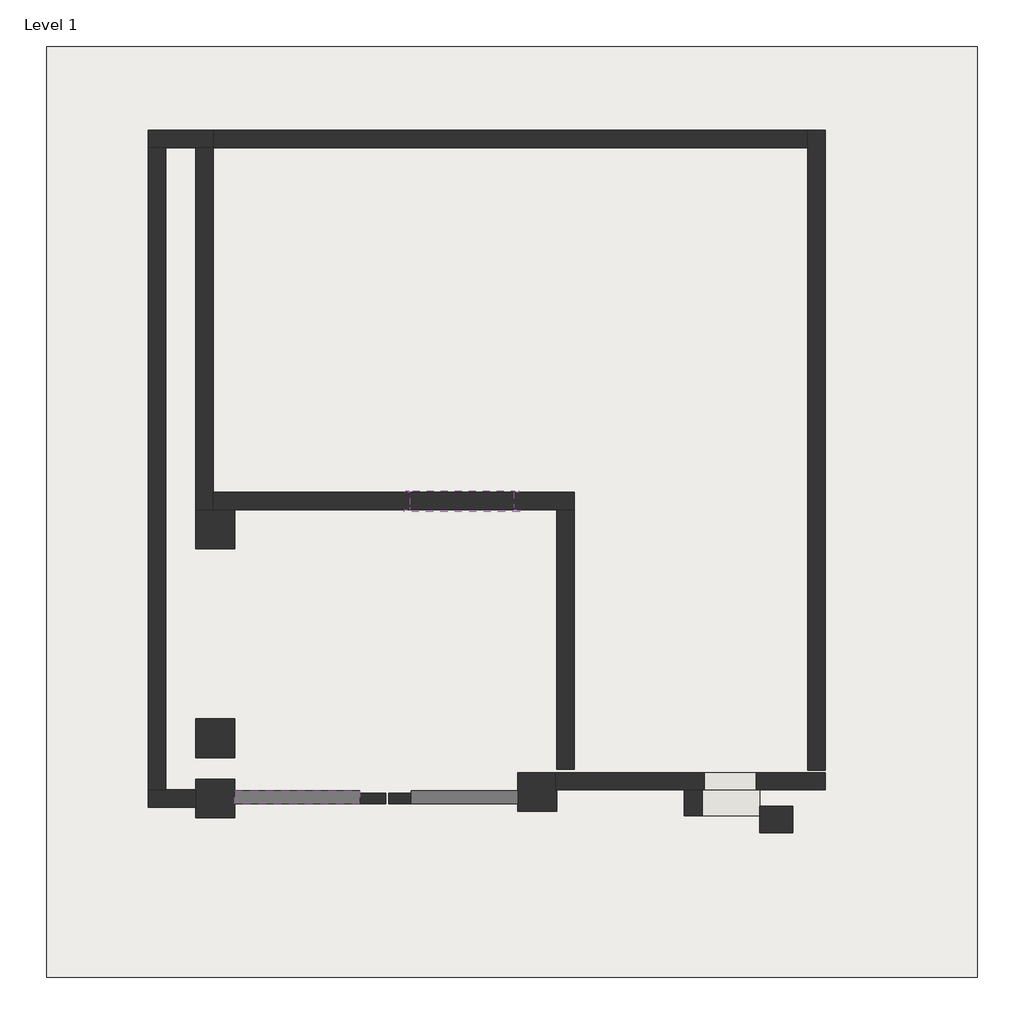
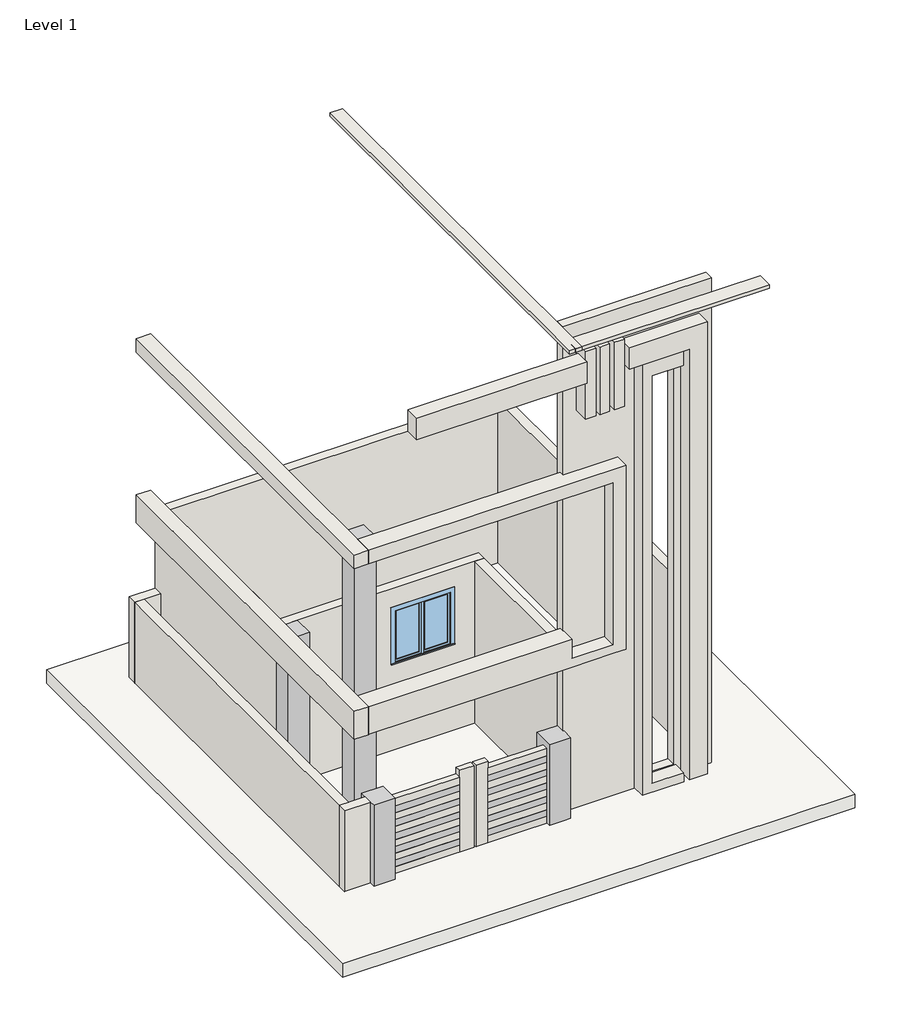
# One storey: 12 walls, 5 proxies, 4 columns, 1 slab, 1 window.
"""IFC4 building model written with IfcOpenShell, lengths in millimetres."""

from ifc_helpers import new_model, si_unit, frame, origin, origin_with_axes, place, context, project, spatial, polyline, outline, extrude, faceted_brep, transform, mapped, element, save
from components import column_b90849dc, walls_1_walls_1_d3114a13, window_0862ab64

model = new_model("IFC4")

# Units and contexts
model_context = context("Model", 3, world=origin())
ifc_project = project(units=[si_unit("LENGTHUNIT", "METRE", prefix="MILLI")], contexts=[model_context])

# Site, building, storey
site = spatial("IfcSite", under=ifc_project)
building = spatial("IfcBuilding", under=site)
storey = spatial("IfcBuildingStorey", under=building, Name="Level 1", Elevation=0.0)

# Proxies
placement = place(None, origin())
element("IfcBuildingElementProxy", 1, Name="Reveal", ObjectType="Reveal", at=placement, inside=storey, context=model_context, shape_type="SweptSolid", body=[
    extrude(outline(polyline([(-7157.3125658, 3805.6483979), (-7157.3125658, 3958.0483979), (-5684.1125658, 3958.0483979), (-5684.1125658, 3805.6483979), (-7157.3125658, 3805.6483979)])), frame((0.0, 0.0, 1371.6), z_axis=(0.0, 0.0, 1.0), x_axis=(1.0, 0.0, 0.0)), (0.0, 0.0, 1.0), 152.4),
    extrude(outline(polyline([(-5074.5125658, 3805.6483979), (-5074.5125658, 3958.0483979), (-3817.2125658, 3958.0483979), (-3817.2125658, 3805.6483979), (-5074.5125658, 3805.6483979)])), frame((0.0, 0.0, 1371.6), z_axis=(0.0, 0.0, 1.0), x_axis=(1.0, 0.0, 0.0)), (0.0, 0.0, 1.0), 152.4),
])
element("IfcBuildingElementProxy", 2, Name="Reveal", ObjectType="Reveal", at=placement, inside=storey, context=model_context, shape_type="SweptSolid", body=[
    extrude(outline(polyline([(-7157.3125658, 3805.6483979), (-7157.3125658, 3958.0483979), (-5684.1125658, 3958.0483979), (-5684.1125658, 3805.6483979), (-7157.3125658, 3805.6483979)])), frame((0.0, 0.0, 1066.8), z_axis=(0.0, 0.0, 1.0), x_axis=(1.0, 0.0, 0.0)), (0.0, 0.0, 1.0), 152.4),
    extrude(outline(polyline([(-5074.5125658, 3805.6483979), (-5074.5125658, 3958.0483979), (-3817.2125658, 3958.0483979), (-3817.2125658, 3805.6483979), (-5074.5125658, 3805.6483979)])), frame((0.0, 0.0, 1066.8), z_axis=(0.0, 0.0, 1.0), x_axis=(1.0, 0.0, 0.0)), (0.0, 0.0, 1.0), 152.4),
])
element("IfcBuildingElementProxy", 3, Name="Reveal", ObjectType="Reveal", at=placement, inside=storey, context=model_context, shape_type="SweptSolid", body=[
    extrude(outline(polyline([(-7157.3125658, 3805.6483979), (-7157.3125658, 3958.0483979), (-5684.1125658, 3958.0483979), (-5684.1125658, 3805.6483979), (-7157.3125658, 3805.6483979)])), frame((0.0, 0.0, 762.0), z_axis=(0.0, 0.0, 1.0), x_axis=(1.0, 0.0, 0.0)), (0.0, 0.0, 1.0), 152.4),
    extrude(outline(polyline([(-5074.5125658, 3805.6483979), (-5074.5125658, 3958.0483979), (-3817.2125658, 3958.0483979), (-3817.2125658, 3805.6483979), (-5074.5125658, 3805.6483979)])), frame((0.0, 0.0, 762.0), z_axis=(0.0, 0.0, 1.0), x_axis=(1.0, 0.0, 0.0)), (0.0, 0.0, 1.0), 152.4),
])
element("IfcBuildingElementProxy", 4, Name="Reveal", ObjectType="Reveal", at=placement, inside=storey, context=model_context, shape_type="SweptSolid", body=[
    extrude(outline(polyline([(-7157.3125658, 3805.6483979), (-7157.3125658, 3958.0483979), (-5684.1125658, 3958.0483979), (-5684.1125658, 3805.6483979), (-7157.3125658, 3805.6483979)])), frame((0.0, 0.0, 457.2), z_axis=(0.0, 0.0, 1.0), x_axis=(1.0, 0.0, 0.0)), (0.0, 0.0, 1.0), 152.4),
    extrude(outline(polyline([(-5074.5125658, 3805.6483979), (-5074.5125658, 3958.0483979), (-3817.2125658, 3958.0483979), (-3817.2125658, 3805.6483979), (-5074.5125658, 3805.6483979)])), frame((0.0, 0.0, 457.2), z_axis=(0.0, 0.0, 1.0), x_axis=(1.0, 0.0, 0.0)), (0.0, 0.0, 1.0), 152.4),
])
element("IfcBuildingElementProxy", 5, Name="Reveal", ObjectType="Reveal", at=placement, inside=storey, context=model_context, shape_type="SweptSolid", body=[
    extrude(outline(polyline([(-7157.3125658, 3805.6483979), (-7157.3125658, 3958.0483979), (-5684.1125658, 3958.0483979), (-5684.1125658, 3805.6483979), (-7157.3125658, 3805.6483979)])), frame((0.0, 0.0, 152.4), z_axis=(0.0, 0.0, 1.0), x_axis=(1.0, 0.0, 0.0)), (0.0, 0.0, 1.0), 152.4),
    extrude(outline(polyline([(-5074.5125658, 3805.6483979), (-5074.5125658, 3958.0483979), (-3817.2125658, 3958.0483979), (-3817.2125658, 3805.6483979), (-5074.5125658, 3805.6483979)])), frame((0.0, 0.0, 152.4), z_axis=(0.0, 0.0, 1.0), x_axis=(1.0, 0.0, 0.0)), (0.0, 0.0, 1.0), 152.4),
])

# Columns
element("IfcColumn", 6, ObjectType="Rectangular Column : 18\" x 18\"", at=placement, inside=storey, context=model_context, shape_type="Brep", body=[
    faceted_brep([(-7157.3125658, 7272.7483979, 3657.6), (-7411.3125658, 7272.7483979, 3657.6), (-7614.5125658, 7272.7483979, 3657.6), (-7614.5125658, 6815.5483979, 3657.6), (-7157.3125658, 6815.5483979, 3657.6), (-7157.3125658, 7272.7483979, 0.0), (-7157.3125658, 6815.5483979, 0.0), (-7614.5125658, 6815.5483979, 0.0), (-7614.5125658, 7272.7483979, 0.0), (-7411.3125658, 7272.7483979, 0.0)], [[[0, 1, 2, 3, 4]], [[5, 6, 7, 8, 9]], [[2, 1, 0, 5, 9, 8]], [[3, 2, 8, 7]], [[4, 3, 7, 6]], [[0, 4, 6, 5]]]),
])
element("IfcColumn", 7, ObjectType="Rectangular Column : 18\" x 18\"", at=placement, inside=storey, context=model_context, shape_type="Brep", body=[
    faceted_brep([(-7157.3125658, 4097.7483979, 1828.8), (-7614.5125658, 4097.7483979, 1828.8), (-7614.5125658, 3970.7483979, 1828.8), (-7614.5125658, 3767.5483979, 1828.8), (-7614.5125658, 3640.5483979, 1828.8), (-7157.3125658, 3640.5483979, 1828.8), (-7157.3125658, 4097.7483979, 0.0), (-7157.3125658, 3932.6483979, 0.0), (-7157.3125658, 3805.6483979, 0.0), (-7157.3125658, 3640.5483979, 0.0), (-7614.5125658, 3640.5483979, 0.0), (-7614.5125658, 3767.5483979, 0.0), (-7614.5125658, 3970.7483979, 0.0), (-7614.5125658, 4097.7483979, 0.0)], [[[0, 1, 2, 3, 4, 5]], [[6, 7, 8, 9, 10, 11, 12, 13]], [[1, 0, 6, 13]], [[4, 3, 2, 1, 13, 12, 11, 10]], [[5, 4, 10, 9]], [[0, 5, 9, 8, 7, 6]]]),
])
element("IfcColumn", 8, ObjectType="Rectangular Column : 18\" x 18\"", at=placement, inside=storey, context=model_context, shape_type="Brep", body=[
    faceted_brep([(-3817.2125658, 4173.9483979, 1828.8), (-3817.2125658, 3716.7483979, 1828.8), (-3360.0125658, 3716.7483979, 1828.8), (-3360.0125658, 3970.7483979, 1828.8), (-3372.7125658, 3970.7483979, 1828.8), (-3372.7125658, 4173.9483979, 1828.8), (-3360.0125658, 3716.7483979, 0.0), (-3817.2125658, 3716.7483979, 0.0), (-3817.2125658, 3805.6483979, 0.0), (-3817.2125658, 3932.6483979, 0.0), (-3817.2125658, 4173.9483979, 0.0), (-3372.7125658, 4173.9483979, 0.0), (-3372.7125658, 3970.7483979, 0.0), (-3360.0125658, 3970.7483979, 0.0)], [[[0, 1, 2, 3, 4, 5]], [[6, 7, 8, 9, 10, 11, 12, 13]], [[10, 0, 5, 11]], [[1, 0, 10, 9, 8, 7]], [[2, 1, 7, 6]], [[2, 6, 13, 3]], [[12, 4, 3, 13]], [[4, 12, 11, 5]]]),
])
column_shape = column_b90849dc(model_context)
element("IfcColumn", 9, ObjectType="Rectangular Column : 18\" x 18\"", at=placement, inside=storey, context=model_context, shape_type="MappedRepresentation", body=[
    mapped(column_shape, transform((-7385.9125658, 4580.3483979, 0.0), x_axis=(1.0, 0.0, 0.0), y_axis=(0.0, 1.0, 0.0), z_axis=(0.0, 0.0, 1.0))),
])

# Slab
element("IfcSlab", 10, ObjectType="Generic - 12\"", at=placement, inside=storey, context=model_context, shape_type="SweptSolid", body=[
    extrude(outline(polyline([(1598.6314273, 12732.6295053), (1598.6314273, 1759.8295053), (-9374.1685727, 1759.8295053), (-9374.1685727, 12732.6295053), (1598.6314273, 12732.6295053)])), frame((0.0, 0.0, -304.8), z_axis=(0.0, 0.0, 1.0), x_axis=(1.0, 0.0, 0.0)), (0.0, 0.0, 1.0), 304.8),
])

# Walls
element("IfcWall", 11, ObjectType="Generic - 5\"", at=placement, inside=storey, context=model_context, shape_type="SweptSolid", body=[
    extrude(outline(polyline([(-3817.2125658, 3805.6483979), (-5074.5125658, 3805.6483979), (-5074.5125658, 3932.6483979), (-3817.2125658, 3932.6483979), (-3817.2125658, 3805.6483979)])), frame((0.0, 0.0, 1524.0), z_axis=(0.0, 0.0, 1.0), x_axis=(1.0, 0.0, 0.0)), (0.0, 0.0, 1.0), 171.4628495),
    extrude(outline(polyline([(-5684.1125658, 3805.6483979), (-7157.3125658, 3805.6483979), (-7157.3125658, 3932.6483979), (-5684.1125658, 3932.6483979), (-5684.1125658, 3805.6483979)])), frame((0.0, 0.0, 1524.0), z_axis=(0.0, 0.0, 1.0), x_axis=(1.0, 0.0, 0.0)), (0.0, 0.0, 1.0), 171.4628495),
    extrude(outline(polyline([(-5684.1125658, 3805.6483979), (-7157.3125658, 3805.6483979), (-7157.3125658, 3932.6483979), (-5684.1125658, 3932.6483979), (-5684.1125658, 3805.6483979)])), frame((0.0, 0.0, 1219.2), z_axis=(0.0, 0.0, 1.0), x_axis=(1.0, 0.0, 0.0)), (0.0, 0.0, 1.0), 152.4),
    extrude(outline(polyline([(-3817.2125658, 3805.6483979), (-5074.5125658, 3805.6483979), (-5074.5125658, 3932.6483979), (-3817.2125658, 3932.6483979), (-3817.2125658, 3805.6483979)])), frame((0.0, 0.0, 1219.2), z_axis=(0.0, 0.0, 1.0), x_axis=(1.0, 0.0, 0.0)), (0.0, 0.0, 1.0), 152.4),
    extrude(outline(polyline([(-5684.1125658, 3805.6483979), (-7157.3125658, 3805.6483979), (-7157.3125658, 3932.6483979), (-5684.1125658, 3932.6483979), (-5684.1125658, 3805.6483979)])), frame((0.0, 0.0, 914.4), z_axis=(0.0, 0.0, 1.0), x_axis=(1.0, 0.0, 0.0)), (0.0, 0.0, 1.0), 152.4),
    extrude(outline(polyline([(-3817.2125658, 3805.6483979), (-5074.5125658, 3805.6483979), (-5074.5125658, 3932.6483979), (-3817.2125658, 3932.6483979), (-3817.2125658, 3805.6483979)])), frame((0.0, 0.0, 914.4), z_axis=(0.0, 0.0, 1.0), x_axis=(1.0, 0.0, 0.0)), (0.0, 0.0, 1.0), 152.4),
    extrude(outline(polyline([(-5684.1125658, 3805.6483979), (-7157.3125658, 3805.6483979), (-7157.3125658, 3932.6483979), (-5684.1125658, 3932.6483979), (-5684.1125658, 3805.6483979)])), frame((0.0, 0.0, 609.6), z_axis=(0.0, 0.0, 1.0), x_axis=(1.0, 0.0, 0.0)), (0.0, 0.0, 1.0), 152.4),
    extrude(outline(polyline([(-3817.2125658, 3805.6483979), (-5074.5125658, 3805.6483979), (-5074.5125658, 3932.6483979), (-3817.2125658, 3932.6483979), (-3817.2125658, 3805.6483979)])), frame((0.0, 0.0, 609.6), z_axis=(0.0, 0.0, 1.0), x_axis=(1.0, 0.0, 0.0)), (0.0, 0.0, 1.0), 152.4),
    extrude(outline(polyline([(-5684.1125658, 3805.6483979), (-7157.3125658, 3805.6483979), (-7157.3125658, 3932.6483979), (-5684.1125658, 3932.6483979), (-5684.1125658, 3805.6483979)])), frame((0.0, 0.0, 304.8), z_axis=(0.0, 0.0, 1.0), x_axis=(1.0, 0.0, 0.0)), (0.0, 0.0, 1.0), 152.4),
    extrude(outline(polyline([(-5684.1125658, 3805.6483979), (-7157.3125658, 3805.6483979), (-7157.3125658, 3932.6483979), (-5684.1125658, 3932.6483979), (-5684.1125658, 3805.6483979)])), origin_with_axes(), (0.0, 0.0, 1.0), 152.4),
    extrude(outline(polyline([(-3817.2125658, 3805.6483979), (-5074.5125658, 3805.6483979), (-5074.5125658, 3932.6483979), (-3817.2125658, 3932.6483979), (-3817.2125658, 3805.6483979)])), origin_with_axes(), (0.0, 0.0, 1.0), 152.4),
    extrude(outline(polyline([(-3817.2125658, 3805.6483979), (-5074.5125658, 3805.6483979), (-5074.5125658, 3932.6483979), (-3817.2125658, 3932.6483979), (-3817.2125658, 3805.6483979)])), frame((0.0, 0.0, 304.8), z_axis=(0.0, 0.0, 1.0), x_axis=(1.0, 0.0, 0.0)), (0.0, 0.0, 1.0), 152.4),
])
element("IfcWall", 12, ObjectType="Generic - 5\"", at=placement, inside=storey, context=model_context, shape_type="Brep", body=[
    faceted_brep([(-5684.1125658, 3805.6483979, 0.0), (-5373.201579, 3805.6483979, 0.0), (-5373.201579, 3805.6483979, 1844.5119599), (-5684.1125658, 3805.6483979, 1844.5119599), (-5684.1125658, 3805.6483979, 1695.4628495), (-5684.1125658, 3805.6483979, 1524.0), (-5684.1125658, 3805.6483979, 1371.6), (-5684.1125658, 3805.6483979, 1219.2), (-5684.1125658, 3805.6483979, 1066.8), (-5684.1125658, 3805.6483979, 914.4), (-5684.1125658, 3805.6483979, 762.0), (-5684.1125658, 3805.6483979, 609.6), (-5684.1125658, 3805.6483979, 457.2), (-5684.1125658, 3805.6483979, 304.8), (-5684.1125658, 3805.6483979, 152.4), (-5684.1125658, 3932.6483979, 0.0), (-5684.1125658, 3932.6483979, 152.4), (-5684.1125658, 3932.6483979, 304.8), (-5684.1125658, 3932.6483979, 457.2), (-5684.1125658, 3932.6483979, 609.6), (-5684.1125658, 3932.6483979, 762.0), (-5684.1125658, 3932.6483979, 914.4), (-5684.1125658, 3932.6483979, 1066.8), (-5684.1125658, 3932.6483979, 1219.2), (-5684.1125658, 3932.6483979, 1371.6), (-5684.1125658, 3932.6483979, 1524.0), (-5684.1125658, 3932.6483979, 1695.4628495), (-5684.1125658, 3932.6483979, 1844.5119599), (-5373.201579, 3932.6483979, 1844.5119599), (-5373.201579, 3932.6483979, 0.0)], [[[0, 1, 2, 3, 4, 5, 6, 7, 8, 9, 10, 11, 12, 13, 14]], [[15, 16, 17, 18, 19, 20, 21, 22, 23, 24, 25, 26, 27, 28, 29]], [[0, 14, 13, 12, 11, 10, 9, 8, 7, 6, 5, 4, 3, 27, 26, 25, 24, 23, 22, 21, 20, 19, 18, 17, 16, 15]], [[1, 0, 15, 29]], [[2, 1, 29, 28]], [[3, 2, 28, 27]]]),
    faceted_brep([(-5074.5125658, 3805.6483979, 1844.5119599), (-5339.2101402, 3805.6483979, 1844.5119599), (-5339.2101402, 3805.6483979, 0.0), (-5074.5125658, 3805.6483979, 0.0), (-5074.5125658, 3805.6483979, 152.4), (-5074.5125658, 3805.6483979, 304.8), (-5074.5125658, 3805.6483979, 457.2), (-5074.5125658, 3805.6483979, 609.6), (-5074.5125658, 3805.6483979, 762.0), (-5074.5125658, 3805.6483979, 914.4), (-5074.5125658, 3805.6483979, 1066.8), (-5074.5125658, 3805.6483979, 1219.2), (-5074.5125658, 3805.6483979, 1371.6), (-5074.5125658, 3805.6483979, 1524.0), (-5074.5125658, 3805.6483979, 1695.4628495), (-5074.5125658, 3932.6483979, 1844.5119599), (-5074.5125658, 3932.6483979, 1695.4628495), (-5074.5125658, 3932.6483979, 1524.0), (-5074.5125658, 3932.6483979, 1371.6), (-5074.5125658, 3932.6483979, 1219.2), (-5074.5125658, 3932.6483979, 1066.8), (-5074.5125658, 3932.6483979, 914.4), (-5074.5125658, 3932.6483979, 762.0), (-5074.5125658, 3932.6483979, 609.6), (-5074.5125658, 3932.6483979, 457.2), (-5074.5125658, 3932.6483979, 304.8), (-5074.5125658, 3932.6483979, 152.4), (-5074.5125658, 3932.6483979, 0.0), (-5339.2101402, 3932.6483979, 0.0), (-5339.2101402, 3932.6483979, 1844.5119599)], [[[0, 1, 2, 3, 4, 5, 6, 7, 8, 9, 10, 11, 12, 13, 14]], [[15, 16, 17, 18, 19, 20, 21, 22, 23, 24, 25, 26, 27, 28, 29]], [[0, 14, 13, 12, 11, 10, 9, 8, 7, 6, 5, 4, 3, 27, 26, 25, 24, 23, 22, 21, 20, 19, 18, 17, 16, 15]], [[1, 0, 15, 29]], [[2, 1, 29, 28]], [[3, 2, 28, 27]]]),
])
element("IfcWall", 13, ObjectType="Generic - 8\"", at=placement, inside=storey, context=model_context, shape_type="Brep", body=[
    faceted_brep([(-7411.3125658, 11539.9483979, 0.0), (-400.9125658, 11539.9483979, 0.0), (-400.9125658, 11539.9483979, 3657.6), (-7411.3125658, 11539.9483979, 3657.6), (-7411.3125658, 11539.9483979, 1828.8), (-7411.3125658, 11743.1483979, 0.0), (-7411.3125658, 11743.1483979, 1828.8), (-7411.3125658, 11743.1483979, 3657.6), (-400.9125658, 11743.1483979, 3657.6), (-400.9125658, 11743.1483979, 0.0)], [[[0, 1, 2, 3, 4]], [[5, 6, 7, 8, 9]], [[1, 0, 5, 9]], [[2, 1, 9, 8]], [[3, 2, 8, 7]], [[0, 4, 3, 7, 6, 5]]]),
])
element("IfcWall", 14, ObjectType="Generic - 8\"", at=placement, inside=storey, context=model_context, shape_type="Brep", body=[
    faceted_brep([(-7411.3125658, 7272.7483979, 0.0), (-7411.3125658, 7475.9483979, 0.0), (-7411.3125658, 11539.9483979, 0.0), (-7411.3125658, 11539.9483979, 1828.8), (-7411.3125658, 11743.1483979, 1828.8), (-7411.3125658, 11743.1483979, 3657.6), (-7411.3125658, 11539.9483979, 3657.6), (-7411.3125658, 7475.9483979, 3657.6), (-7411.3125658, 7272.7483979, 3657.6), (-7614.5125658, 7272.7483979, 0.0), (-7614.5125658, 7272.7483979, 3657.6), (-7614.5125658, 11743.1483979, 3657.6), (-7614.5125658, 11743.1483979, 1828.8), (-7614.5125658, 11539.9483979, 1828.8), (-7614.5125658, 11539.9483979, 0.0)], [[[0, 1, 2, 3, 4, 5, 6, 7, 8]], [[9, 10, 11, 12, 13, 14]], [[2, 1, 0, 9, 14]], [[8, 7, 6, 5, 11, 10]], [[0, 8, 10, 9]], [[12, 4, 3, 13]], [[3, 2, 14, 13]], [[5, 4, 12, 11]]]),
])
element("IfcWall", 15, ObjectType="Generic - 8\"", at=placement, inside=storey, context=model_context, shape_type="Brep", body=[
    faceted_brep([(-400.9125658, 11743.1483979, 0.0), (-400.9125658, 11539.9483979, 0.0), (-400.9125658, 4199.3483979, 0.0), (-400.9125658, 4199.3483979, 3657.6), (-400.9125658, 4275.5483979, 3657.6), (-400.9125658, 11539.9483979, 3657.6), (-400.9125658, 11743.1483979, 3657.6), (-197.7125658, 11743.1483979, 0.0), (-197.7125658, 11743.1483979, 3657.6), (-197.7125658, 4275.5483979, 3657.6), (-197.7125658, 4199.3483979, 3657.6), (-197.7125658, 4199.3483979, 0.0)], [[[0, 1, 2, 3, 4, 5, 6]], [[7, 8, 9, 10, 11]], [[2, 1, 0, 7, 11]], [[3, 2, 11, 10]], [[0, 6, 8, 7]], [[4, 3, 10, 9]], [[6, 5, 4, 9, 8]]]),
])
element("IfcWall", 16, ObjectType="Generic - 8\"", at=placement, inside=storey, context=model_context, shape_type="Brep", body=[
    faceted_brep([(-7411.3125658, 7272.7483979, 0.0), (-7157.3125658, 7272.7483979, 0.0), (-3360.0125658, 7272.7483979, 0.0), (-3156.8125658, 7272.7483979, 0.0), (-3156.8125658, 7272.7483979, 3657.6), (-3360.0125658, 7272.7483979, 3657.6), (-7157.3125658, 7272.7483979, 3657.6), (-7411.3125658, 7272.7483979, 3657.6), (-5087.2125658, 7272.7483979, 3171.7508635), (-3868.0125658, 7272.7483979, 3171.7508635), (-3868.0125658, 7272.7483979, 1952.5508635), (-5087.2125658, 7272.7483979, 1952.5508635), (-7411.3125658, 7475.9483979, 0.0), (-7411.3125658, 7475.9483979, 3657.6), (-3156.8125658, 7475.9483979, 3657.6), (-3156.8125658, 7475.9483979, 0.0), (-5087.2125658, 7475.9483979, 3171.7508635), (-5087.2125658, 7475.9483979, 1952.5508635), (-3868.0125658, 7475.9483979, 1952.5508635), (-3868.0125658, 7475.9483979, 3171.7508635)], [[[0, 1, 2, 3, 4, 5, 6, 7], [8, 9, 10, 11]], [[12, 13, 14, 15], [16, 17, 18, 19]], [[3, 2, 1, 0, 12, 15]], [[0, 7, 13, 12]], [[4, 3, 15, 14]], [[7, 6, 5, 4, 14, 13]], [[17, 16, 8, 11]], [[18, 17, 11, 10]], [[19, 18, 10, 9]], [[16, 19, 9, 8]]]),
])
element("IfcWall", 17, ObjectType="Generic - 8\"", at=placement, inside=storey, context=model_context, shape_type="SweptSolid", body=[
    extrude(outline(polyline([(7272.7483979, 0.0), (4212.0483979, 0.0), (4212.0483979, 3657.6), (4275.5483979, 3657.6), (7272.7483979, 3657.6), (7272.7483979, 0.0)])), frame((-3360.0125658, 0.0, 0.0), z_axis=(1.0, 0.0, 0.0), x_axis=(0.0, 1.0, 0.0)), (0.0, 0.0, 1.0), 203.2),
])
element("IfcWall", 18, ObjectType="Generic - 8\"", at=placement, inside=storey, context=model_context, shape_type="Brep", body=[
    faceted_brep([(-3372.7125658, 3970.7483979, 0.0), (-3360.0125658, 3970.7483979, 0.0), (-197.7125658, 3970.7483979, 0.0), (-197.7125658, 3970.7483979, 10972.8), (-3372.7125658, 3970.7483979, 10972.8), (-3372.7125658, 3970.7483979, 1828.8), (-1620.1125658, 3970.7483979, 9398.0), (-1010.5125658, 3970.7483979, 9398.0), (-1010.5125658, 3970.7483979, 254.0), (-1620.1125658, 3970.7483979, 254.0), (-3372.7125658, 4173.9483979, 0.0), (-3372.7125658, 4173.9483979, 1828.8), (-3372.7125658, 4173.9483979, 10972.8), (-197.7125658, 4173.9483979, 10972.8), (-197.7125658, 4173.9483979, 0.0), (-1620.1125658, 4173.9483979, 9398.0), (-1620.1125658, 4173.9483979, 254.0), (-1010.5125658, 4173.9483979, 254.0), (-1010.5125658, 4173.9483979, 9398.0)], [[[0, 1, 2, 3, 4, 5], [6, 7, 8, 9]], [[10, 11, 12, 13, 14], [15, 16, 17, 18]], [[2, 1, 0, 10, 14]], [[3, 2, 14, 13]], [[0, 5, 4, 12, 11, 10]], [[4, 3, 13, 12]], [[16, 15, 6, 9]], [[17, 16, 9, 8]], [[18, 17, 8, 7]], [[15, 18, 7, 6]]]),
])
element("IfcWall", 19, ObjectType="Generic - 8\"", at=placement, inside=storey, context=model_context, shape_type="SweptSolid", body=[
    extrude(outline(polyline([(-8173.3125658, 3970.7483979), (-8173.3125658, 11539.9483979), (-7970.1125658, 11539.9483979), (-7970.1125658, 3970.7483979), (-8173.3125658, 3970.7483979)])), origin_with_axes(), (0.0, 0.0, 1.0), 1828.8),
])
element("IfcWall", 20, ObjectType="Generic - 8\"", at=placement, inside=storey, context=model_context, shape_type="Brep", body=[
    faceted_brep([(-8173.3125658, 11539.9483979, 0.0), (-7970.1125658, 11539.9483979, 0.0), (-7614.5125658, 11539.9483979, 0.0), (-7411.3125658, 11539.9483979, 0.0), (-7411.3125658, 11539.9483979, 1828.8), (-7614.5125658, 11539.9483979, 1828.8), (-7970.1125658, 11539.9483979, 1828.8), (-8173.3125658, 11539.9483979, 1828.8), (-8173.3125658, 11743.1483979, 0.0), (-8173.3125658, 11743.1483979, 1828.8), (-7614.5125658, 11743.1483979, 1828.8), (-7411.3125658, 11743.1483979, 1828.8), (-7411.3125658, 11743.1483979, 0.0)], [[[0, 1, 2, 3, 4, 5, 6, 7]], [[8, 9, 10, 11, 12]], [[3, 2, 1, 0, 8, 12]], [[7, 6, 5, 4, 11, 10, 9]], [[0, 7, 9, 8]], [[4, 3, 12, 11]]]),
])
element("IfcWall", 21, ObjectType="Generic - 8\"", at=placement, inside=storey, context=model_context, shape_type="Brep", body=[
    faceted_brep([(-8173.3125658, 3767.5483979, 0.0), (-7614.5125658, 3767.5483979, 0.0), (-7614.5125658, 3767.5483979, 1828.8), (-8173.3125658, 3767.5483979, 1828.8), (-8173.3125658, 3970.7483979, 0.0), (-8173.3125658, 3970.7483979, 1828.8), (-7970.1125658, 3970.7483979, 1828.8), (-7614.5125658, 3970.7483979, 1828.8), (-7614.5125658, 3970.7483979, 0.0), (-7970.1125658, 3970.7483979, 0.0)], [[[0, 1, 2, 3]], [[4, 5, 6, 7, 8, 9]], [[1, 0, 4, 9, 8]], [[2, 1, 8, 7]], [[3, 2, 7, 6, 5]], [[0, 3, 5, 4]]]),
])
walls_1_walls_1_shape = walls_1_walls_1_d3114a13(model_context)
element("IfcWall", 22, ObjectType="Walls 1 : Walls 1", at=placement, inside=storey, context=model_context, shape_type="MappedRepresentation", body=[
    mapped(walls_1_walls_1_shape, transform((0.0, 0.0, 0.0), x_axis=(1.0, 0.0, 0.0), y_axis=(0.0, 1.0, 0.0), z_axis=(0.0, 0.0, 1.0))),
])

# Window
window_shape = window_0862ab64(model_context)
element("IfcWindow", 23, ObjectType="Casement Dbl with Trim : 48\" x 48\"", at=placement, inside=storey, context=model_context, shape_type="MappedRepresentation", body=[
    mapped(window_shape, transform((-4477.6125658, 7393.3983979, 1038.1508635), x_axis=(-1.0, 0.0, 0.0), y_axis=(0.0, -1.0, 0.0), z_axis=(0.0, 0.0, 1.0))),
])

save(model, "model.ifc")

# Revit data of these elements
# Type "Rectangular Column : 18\" x 18\""
#   Assembly Code = "B1010200"
#   Depth = 1' - 6"
#   Offset Base = 0' - 0"
#   Offset Top = 0' - 0"
#   Width = 1' - 6"
#   Material = none
# Type "Generic - 12\""
#   Assembly Code = "B1010"
#   Function = 0
#   Layers, outside or top first: 1' - 0" no material (function 1)
# Type "Generic - 5\""
#   Assembly Code = "B2010"
#   Layers, outside or top first: 0' - 5" no material (function 1)
# Type "Generic - 8\""
#   Assembly Code = "B2010"
#   Layers, outside or top first: 0' - 8" no material (function 1)
# Type "Casement Dbl with Trim : 48\" x 48\""
#   Type Mark = "13"
#   Construction Type Id = "GSP4R"
#   Assembly Code = "B2020100"
#   Analytic Construction = "1/8 in Pilkington single glazing"
#   Visual Light Transmittance = 0.9
#   Solar Heat Gain Coefficient = 0.78
#   Heat Transfer Coefficient (U) = 0.6496 BTU/(h·ft²·°F)
#   Height = 4' - 0"
#   Default Sill Height = 3' - 0"
#   Trim Projection - Ext. = 0' - 0 1/2"
#   Trim Projection - Int. = 0' - 0 3/4"
#   Trim Width - Exterior = 0' - 3 1/2"
#   Trim Width - Interior = 0' - 3 1/2"
#   Width = 4' - 0"
#   Window Inset = 0' - 0 3/4"
#   Define Thermal Properties by = 1
#   Glass Pane Material = Glass
#   Sash Material = Sash
#   Trim Exterior Material = Trim
#   Trim Interior Material = Trim
#   Wall Closure = (empty or 0)
# Elements 6, 7, 8 (IfcColumn, "Rectangular Column : 18\" x 18\"")
#   Phase Created = New Construction
#   Materials on its faces: "Default Wall"
# Element 9 (IfcColumn, "Rectangular Column : 18\" x 18\"")
#   Phase Created = New Construction
# Element 10 (IfcSlab, "Generic - 12\"")
#   Height Offset From Level = 0' - 0"
#   Phase Created = New Construction
#   Materials on its faces: "Default Floor"
# Element 11 (IfcWall, "Generic - 5\"")
#   Top Offset = -6' - 5.24949"
#   Base Offset = 0' - 0"
#   wall height = 5' - 6.75051"
#   Phase Created = New Construction
#   Base Constraint = Level 1
#   Top Constraint = Level 2
#   Materials on its faces: "Default Wall"
# Element 12 (IfcWall, "Generic - 5\"")
#   Top Offset = -5' - 11.38142"
#   Base Offset = 0' - 0"
#   wall height = 6' - 0.61858"
#   Phase Created = New Construction
#   Base Constraint = Level 1
#   Top Constraint = Level 2
#   Materials on its faces: "Default Wall"
# Elements 13, 14, 15, 16, 17 (IfcWall, "Generic - 8\"")
#   Top Offset = 0' - 0"
#   Base Offset = 0' - 0"
#   Unconnected Height = 12' - 0"
#   wall height = 12' - 0"
#   Phase Created = New Construction
#   Base Constraint = Level 1
#   Materials on its faces: "Default Wall"
# Element 18 (IfcWall, "Generic - 8\"")
#   Top Offset = 0' - 0"
#   Base Offset = 0' - 0"
#   Unconnected Height = 36' - 0"
#   wall height = 36' - 0"
#   Phase Created = New Construction
#   Base Constraint = Level 1
#   Materials on its faces: "Default Wall"
# Elements 19, 20, 21 (IfcWall, "Generic - 8\"")
#   Top Offset = 0' - 0"
#   Base Offset = 0' - 0"
#   Unconnected Height = 6' - 0"
#   wall height = 6' - 0"
#   Phase Created = New Construction
#   Base Constraint = Level 1
#   Materials on its faces: "Default Wall"
# Element 22 (IfcWall, "Walls 1 : Walls 1")
#   Phase Created = New Construction
#   Materials on its faces: "Default Wall"
# Element 23 (IfcWindow, "Casement Dbl with Trim : 48\" x 48\"")
#   Mark = "2"
#   Phase Created = New Construction
#   Materials on its faces: "Sash", "Trim", "Glass"
# Materials
#   "Glass": class "Glass", colour RGB 0 128 192, transparency 0.75, Description = "Soda Lime Glass", Cost = 0
#   "Sash": class "Wood", colour RGB 224 178 126, transparency 0
#   "Trim": class "Wood", colour RGB 224 178 126, transparency 0
#   "Default Wall": colour RGB 128 128 128, transparency 0
#   "Default Floor": colour RGB 128 128 128, transparency 0
